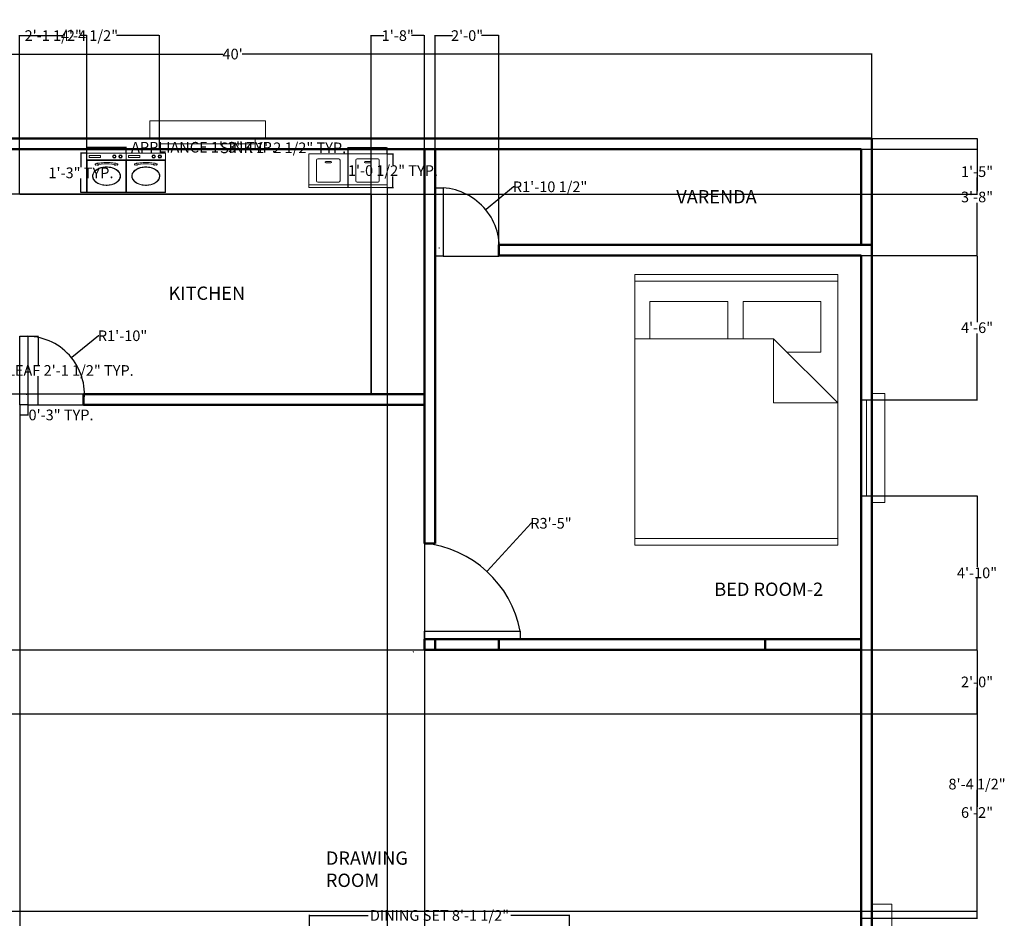
# Model space of a CAD drawing. Units: inches. Extents: x 749 to 1356, y 222 to 907.
# Tile 4 of 4: x 981 to 1351, y 570 to 907. Entities that reach past the tile are written whole.
import ezdxf

# ---------------------------------------------------------------- set-up
doc = ezdxf.new("R2010")
doc.units = ezdxf.units.IN
doc.header["$MEASUREMENT"] = 0
for name, color, linetype, lineweight in [('A-ANNO-DIMS', 30, 'Continuous', 18), ('A-AREA-IDEN', 6, 'Continuous', 25), ('A-EQPM', 8, 'Continuous', 18), ('A-FLOR-CASE', 34, 'Continuous', 25), ('A-FLOR-FIXT', 9, 'Continuous', 18), ('A-GLAZ', 4, 'Continuous', 20), ('A-WALL', 7, 'Continuous', 50), ('DOOR', 4, 'Continuous', 25), ('FURNITURE', 32, 'Continuous', 18)]:
    doc.layers.add(name, color=color, linetype=linetype, lineweight=lineweight)
doc.styles.get("Standard").update_dxf_attribs({"font": 'arial.ttf'})
doc.dimstyles.get("Standard").update_dxf_attribs({"dimtxt": 4, "dimasz": 0.18, "dimexe": 0.18, "dimexo": 0.0625, "dimgap": 0.09, "dimtad": 0, "dimtih": 1, "dimtoh": 1, "dimdec": 0, "dimrnd": 6, "dimzin": 0, "dimdsep": 46, "dimlunit": 3, "dimtxsty": 'Standard', "dimcen": 0.09, "dimadec": 0, "dimazin": 0, "dimtfac": 1, "dimtdec": 0, "dimtofl": 0, "dimtmove": 0, "dimatfit": 3, "dimfxl": 1, "dimtolj": 1, "dimtzin": 0, "dimarcsym": 0})

# ---------------------------------------------------------------- blocks, each defined once
blk = doc.blocks.new('QUEEN-00')
for p, q in [((-0.8475, -0.7751), (-0.8475, 0.7489)), ((0.6511, 0.7489), (0.6511, -0.2925)), ((1.0829, 0.7489), (1.0829, -0.7751)), ((0.9305, 0.6346), (0.6511, 0.6346)), ((0.9305, 0.0504), (0.9305, 0.6346)), ((0.6511, 0.0504), (0.9305, 0.0504)), ((0.9305, -0.0639), (0.6511, -0.0639)), ((0.9305, -0.6481), (0.9305, -0.0639)), ((0.1685, -0.7751), (0.6511, -0.2925)), ((0.1685, -0.2925), (0.1685, -0.7751)), ((0.6511, -0.2925), (0.1685, -0.2925)), ((0.5495, -0.3941), (0.5495, -0.6481)), ((0.5495, -0.6481), (0.9305, -0.6481))]:
    blk.add_line(p, q)
blk.add_lwpolyline([(-0.8983, -0.7751), (-0.8983, 0.7489), (1.1337, 0.7489), (1.1337, -0.7751)], close=True)
blk = doc.blocks.new('A$C7E884C79')
for p, q in [((0, 0), (0, 600)), ((0, 600), (0, 0)), ((0, 600), (600, 600)), ((600, 500), (0, 500)), ((600, 495), (0, 495)), ((600, 600), (600, 0)), ((600, 0), (600, 600)), ((600, 600), (600, 450)), ((600, 600), (600, 500)), ((600, 500), (600, 0)), ((0, 0), (600, 0))]:
    blk.add_line(p, q)
for points in [[(5, 490), (595, 490), (595, 5), (5, 5)], [(36, 565), (209, 565), (209, 535), (36, 535)]]:
    blk.add_lwpolyline(points, close=True)
for centre, radius in [((419, 550), 27), ((419, 550), 17), ((514, 550), 27), ((514, 550), 17)]:
    blk.add_circle(centre, radius)
for centre, radius, start, end in [((137, 428), 10, 107.9829, 276.9581), ((168, 434), 15, 50.7888, 150.367), ((168, 434), 15, 234.0165, 327.1412), ((432, 434), 15, 212.8588, 305.9835), ((432, 434), 15, 29.633, 129.2112), ((463, 428), 10, 263.0419, 72.0171)]:
    blk.add_arc(centre, radius, start, end)
blk.add_ellipse((300, 250), major_axis=(-210, 0), ratio=0.648352)
for points, knots in [([(134, 437), (145, 440), (155, 442), (186, 447), (206, 451), (248, 456), (269, 458), (294, 459), (297, 459), (305, 459), (308, 459), (320, 459), (327, 458), (349, 457), (364, 455), (400, 450), (421, 446), (450, 441), (458, 439), (466, 437)], [0, 0, 0, 0, 31.638865, 31.638865, 92.600143, 92.600143, 153.561421, 153.561421, 164.367647, 164.367647, 175.173874, 175.173874, 196.786327, 196.786327, 240.011233, 240.011233, 302.099201, 302.099201, 326.773065, 326.773065, 326.773065, 326.773065]), ([(85, 250), (85, 245), (86, 240), (88, 227), (90, 219), (96, 205), (100, 198), (110, 184), (116, 177), (128, 165), (135, 159), (151, 148), (159, 143), (177, 134), (187, 130), (206, 123), (217, 120), (238, 115), (249, 113), (271, 110), (282, 109), (305, 109), (316, 109), (339, 111), (350, 113), (372, 117), (382, 120), (403, 126), (412, 130), (431, 138), (440, 143), (456, 153), (464, 159), (478, 170), (484, 177), (495, 190), (499, 197), (507, 211), (510, 219), (513, 234), (514, 241), (515, 256), (514, 264), (510, 279), (508, 287), (500, 301), (496, 308), (486, 321), (480, 328), (466, 340), (459, 345), (442, 356), (434, 361), (415, 369), (405, 373), (385, 380), (375, 382), (353, 387), (342, 388), (320, 390), (308, 391), (286, 391), (275, 390), (252, 388), (241, 386), (220, 381), (209, 378), (189, 371), (180, 367), (162, 358), (153, 353), (138, 342), (130, 337), (117, 324), (112, 318), (102, 304), (98, 297), (91, 283), (89, 275), (86, 262), (85, 256), (85, 250)], [0, 0, 0, 0, 0.108301, 0.108301, 0.267534, 0.267534, 0.426768, 0.426768, 0.586002, 0.586002, 0.745235, 0.745235, 0.904469, 0.904469, 1.063703, 1.063703, 1.222936, 1.222936, 1.38217, 1.38217, 1.541404, 1.541404, 1.700637, 1.700637, 1.859871, 1.859871, 2.019105, 2.019105, 2.178339, 2.178339, 2.337572, 2.337572, 2.496806, 2.496806, 2.65604, 2.65604, 2.815273, 2.815273, 2.974507, 2.974507, 3.133741, 3.133741, 3.292974, 3.292974, 3.452208, 3.452208, 3.611442, 3.611442, 3.770676, 3.770676, 3.929909, 3.929909, 4.089143, 4.089143, 4.248377, 4.248377, 4.40761, 4.40761, 4.566844, 4.566844, 4.726078, 4.726078, 4.885311, 4.885311, 5.044545, 5.044545, 5.203779, 5.203779, 5.363012, 5.363012, 5.522246, 5.522246, 5.68148, 5.68148, 5.840714, 5.840714, 5.999947, 5.999947, 6.159181, 6.159181, 6.283185, 6.283185, 6.283185, 6.283185])]:
    blk.add_open_spline(points, degree=3, knots=knots)
blk.add_open_spline([(138, 418), (192, 428), (300, 449), (408, 428), (462, 418)], degree=3)
blk = doc.blocks.new('LAVAD-01')
for p, q in [((-0.322, 0.358), (-0.322, -0.392)), ((0.328, 0.358), (-0.322, 0.358)), ((-0.272, 0.358), (-0.272, -0.392)), ((0.203, 0.208), (-0.197, 0.208)), ((0.328, -0.392), (0.328, 0.358)), ((-0.222, 0.183), (-0.222, -0.217)), ((0.153, 0.033), (0.153, -0.067)), ((0.165, 0.046), (0.165, 0.046)), ((0.178, -0.067), (0.178, 0.033)), ((0.228, -0.217), (0.228, 0.183)), ((0.165, -0.079), (0.165, -0.079)), ((-0.197, -0.242), (0.203, -0.242)), ((-0.322, -0.392), (0.328, -0.392))]:
    blk.add_line(p, q)
for centre, radius, start, end in [((-0.197, 0.183), 0.025, 90, 180), ((0.203, 0.183), 0.025, 0, 90), ((0.165, 0.033), 0.0125, 90, 180), ((0.165, 0.033), 0.0125, 0, 90), ((0.165, -0.067), 0.0125, 180, 270), ((0.165, -0.067), 0.0125, 270, 360), ((-0.197, -0.217), 0.025, 180, 270), ((0.203, -0.217), 0.025, 270, 360)]:
    blk.add_arc(centre, radius, start, end)
blk = doc.blocks.new('*D129')
at = {"layer": 'A-ANNO-DIMS', "color": 0, "lineweight": -2, "transparency": 16777216}
for p, q in [((820.88, 858.33), (820.88, 894.09)), ((821.06, 893.91), (1057.31, 893.91)), ((1300.7, 893.91), (1064.44, 893.91)), ((1300.88, 862.33), (1300.88, 894.09))]:
    blk.add_line(p, q, dxfattribs=at)
at = {"layer": 'A-ANNO-DIMS', "color": 0, "transparency": 16777216}
for points in [[(821.06, 893.94), (821.06, 893.88), (820.88, 893.91)], [(1300.7, 893.94), (1300.7, 893.88), (1300.88, 893.91)]]:
    blk.add_solid(points, dxfattribs=at)
at = {"layer": 'Defpoints', "color": 0, "transparency": 16777216}
for p in [(1300.88, 893.91), (1300.88, 862.27), (820.88, 858.27)]:
    blk.add_point(p, dxfattribs=at)
at = {"layer": 'A-ANNO-DIMS', "color": 0, "transparency": 16777216, "insert": (1060.88, 893.91), "char_height": 4, "attachment_point": 5}
blk.add_mtext("\\A1;40'", dxfattribs=at)
blk = doc.blocks.new('WIN-36IN')
blk.add_lwpolyline([(0, 0), (0, 36), (4, 36), (4, 0)], close=True)
blk.add_lwpolyline([(4, 0), (2.02, 0), (2.02, 36)])
blk = doc.blocks.new('DOOR-LEAF-36IN')
blk.add_lwpolyline([(0, 3), (36, 3), (36, 0), (0, 0)], close=True)
blk = doc.blocks.new('DOOR-LEAF-NARROW')
blk.add_line((0, 25.67), (3, 25.67))
blk.add_lwpolyline([(3, 25.67), (3, 0), (0, 0), (0, 25.67)])
blk = doc.blocks.new('*D141')
at = {"layer": 'A-ANNO-DIMS', "color": 0, "lineweight": -2, "transparency": 16777216}
for p, q in [((984.05, 787.99), (988.01, 787.99)), ((987.83, 787.81), (987.83, 777.32)), ((987.83, 762.5), (987.83, 773)), ((984.05, 762.32), (988.01, 762.32))]:
    blk.add_line(p, q, dxfattribs=at)
at = {"layer": 'A-ANNO-DIMS', "color": 0, "transparency": 16777216}
for points in [[(987.8, 787.81), (987.86, 787.81), (987.83, 787.99)], [(987.8, 762.5), (987.86, 762.5), (987.83, 762.32)]]:
    blk.add_solid(points, dxfattribs=at)
at = {"layer": 'Defpoints', "color": 0, "transparency": 16777216}
for p in [(983.98, 787.99), (987.83, 787.99), (983.98, 762.32)]:
    blk.add_point(p, dxfattribs=at)
at = {"layer": 'A-ANNO-DIMS', "color": 0, "transparency": 16777216, "insert": (987.83, 775.16), "char_height": 4, "attachment_point": 5}
blk.add_mtext('\\A1;NARROW LEAF 2\'-1 1/2" TYP.', dxfattribs=at)
blk = doc.blocks.new('*D142')
at = {"layer": 'A-ANNO-DIMS', "color": 0, "lineweight": -2, "transparency": 16777216}
for p, q in [((980.98, 762.26), (980.98, 758.29)), ((983.98, 762.26), (983.98, 758.29)), ((981.16, 758.47), (983.8, 758.47)), ((983.98, 758.47), (984.16, 758.47))]:
    blk.add_line(p, q, dxfattribs=at)
at = {"layer": 'A-ANNO-DIMS', "color": 0, "transparency": 16777216}
for points in [[(981.16, 758.5), (981.16, 758.44), (980.98, 758.47)], [(983.8, 758.5), (983.8, 758.44), (983.98, 758.47)]]:
    blk.add_solid(points, dxfattribs=at)
at = {"layer": 'Defpoints', "color": 0, "transparency": 16777216}
for p in [(980.98, 762.32), (983.98, 762.32), (983.98, 758.47)]:
    blk.add_point(p, dxfattribs=at)
at = {"layer": 'A-ANNO-DIMS', "color": 0, "transparency": 16777216, "insert": (996.45, 758.47), "char_height": 4, "attachment_point": 5}
blk.add_mtext('\\A1;0\'-3" TYP.', dxfattribs=at)
blk = doc.blocks.new('*D145')
at = {"layer": 'A-ANNO-DIMS', "color": 0, "lineweight": -2, "transparency": 16777216}
for p, q in [((1104.24, 858.72), (1104.06, 858.72)), ((1104.24, 856.58), (1104.24, 858.9)), ((1118.7, 858.72), (1104.42, 858.72)), ((1118.88, 856.58), (1118.88, 858.9))]:
    blk.add_line(p, q, dxfattribs=at)
at = {"layer": 'A-ANNO-DIMS', "color": 0, "transparency": 16777216}
for points in [[(1104.42, 858.75), (1104.42, 858.69), (1104.24, 858.72)], [(1118.7, 858.75), (1118.7, 858.69), (1118.88, 858.72)]]:
    blk.add_solid(points, dxfattribs=at)
at = {"layer": 'Defpoints', "color": 0, "transparency": 16777216}
for p in [(1104.24, 858.72), (1104.24, 856.52), (1118.88, 856.52)]:
    blk.add_point(p, dxfattribs=at)
at = {"layer": 'A-ANNO-DIMS', "color": 0, "transparency": 16777216, "insert": (1079.83, 858.72), "char_height": 4, "attachment_point": 5}
blk.add_mtext('\\A1;SINK 1\'-2 1/2" TYP.', dxfattribs=at)
blk = doc.blocks.new('*D146')
at = {"layer": 'A-ANNO-DIMS', "color": 0, "lineweight": -2, "transparency": 16777216}
for p, q in [((1118.95, 856.52), (1121.26, 856.52)), ((1121.08, 856.34), (1121.08, 852.34)), ((1121.08, 844.01), (1121.08, 848.02)), ((1118.95, 843.83), (1121.26, 843.83))]:
    blk.add_line(p, q, dxfattribs=at)
at = {"layer": 'A-ANNO-DIMS', "color": 0, "transparency": 16777216}
for points in [[(1121.05, 856.34), (1121.11, 856.34), (1121.08, 856.52)], [(1121.05, 844.01), (1121.11, 844.01), (1121.08, 843.83)]]:
    blk.add_solid(points, dxfattribs=at)
at = {"layer": 'Defpoints', "color": 0, "transparency": 16777216}
for p in [(1118.88, 856.52), (1121.08, 856.52), (1118.88, 843.83)]:
    blk.add_point(p, dxfattribs=at)
at = {"layer": 'A-ANNO-DIMS', "color": 0, "transparency": 16777216, "insert": (1121.08, 850.18), "char_height": 4, "attachment_point": 5}
blk.add_mtext('\\A1;1\'-0 1/2" TYP.', dxfattribs=at)
blk = doc.blocks.new('*D149')
at = {"layer": 'A-ANNO-DIMS', "color": 0, "lineweight": -2, "transparency": 16777216}
for p, q in [((1006.14, 856.78), (1006.14, 859.11)), ((1006.32, 858.93), (1020.72, 858.93)), ((1020.9, 856.78), (1020.9, 859.11)), ((1020.9, 858.93), (1021.08, 858.93))]:
    blk.add_line(p, q, dxfattribs=at)
at = {"layer": 'A-ANNO-DIMS', "color": 0, "transparency": 16777216}
for points in [[(1006.32, 858.96), (1006.32, 858.9), (1006.14, 858.93)], [(1020.72, 858.96), (1020.72, 858.9), (1020.9, 858.93)]]:
    blk.add_solid(points, dxfattribs=at)
at = {"layer": 'Defpoints', "color": 0, "transparency": 16777216}
for p in [(1020.9, 858.93), (1006.14, 856.71), (1020.9, 856.71)]:
    blk.add_point(p, dxfattribs=at)
at = {"layer": 'A-ANNO-DIMS', "color": 0, "transparency": 16777216, "insert": (1049.94, 858.93), "char_height": 4, "attachment_point": 5}
blk.add_mtext('\\A1;APPLIANCE 1\'-3" TYP.', dxfattribs=at)
blk = doc.blocks.new('*D150')
at = {"layer": 'A-ANNO-DIMS', "color": 0, "lineweight": -2, "transparency": 16777216}
for p, q in [((1006.08, 856.71), (1003.75, 856.71)), ((1003.93, 856.53), (1003.93, 851.47)), ((1003.93, 842.13), (1003.93, 847.2)), ((1006.08, 841.95), (1003.75, 841.95))]:
    blk.add_line(p, q, dxfattribs=at)
at = {"layer": 'A-ANNO-DIMS', "color": 0, "transparency": 16777216}
for points in [[(1003.9, 856.53), (1003.96, 856.53), (1003.93, 856.71)], [(1003.9, 842.13), (1003.96, 842.13), (1003.93, 841.95)]]:
    blk.add_solid(points, dxfattribs=at)
at = {"layer": 'Defpoints', "color": 0, "transparency": 16777216}
for p in [(1003.93, 856.71), (1006.14, 856.71), (1006.14, 841.95)]:
    blk.add_point(p, dxfattribs=at)
at = {"layer": 'A-ANNO-DIMS', "color": 0, "transparency": 16777216, "insert": (1003.93, 849.33), "char_height": 4, "attachment_point": 5}
blk.add_mtext('\\A1;1\'-3" TYP.', dxfattribs=at)
blk = doc.blocks.new('*D151')
at = {"layer": 'A-ANNO-DIMS', "color": 0, "lineweight": -2, "transparency": 16777216}
for p, q in [((1089.75, 556.06), (1089.75, 570.82)), ((1089.93, 570.64), (1111.83, 570.64)), ((1187.2, 570.64), (1165.29, 570.64)), ((1187.38, 556.06), (1187.38, 570.82))]:
    blk.add_line(p, q, dxfattribs=at)
at = {"layer": 'A-ANNO-DIMS', "color": 0, "transparency": 16777216}
for points in [[(1089.93, 570.67), (1089.93, 570.61), (1089.75, 570.64)], [(1187.2, 570.67), (1187.2, 570.61), (1187.38, 570.64)]]:
    blk.add_solid(points, dxfattribs=at)
at = {"layer": 'Defpoints', "color": 0, "transparency": 16777216}
for p in [(1187.38, 570.64), (1089.75, 556), (1187.38, 556)]:
    blk.add_point(p, dxfattribs=at)
at = {"layer": 'A-ANNO-DIMS', "color": 0, "transparency": 16777216, "insert": (1138.56, 570.64), "char_height": 4, "attachment_point": 5}
blk.add_mtext('\\A1;DINING SET 8\'-1 1/2"', dxfattribs=at)
blk = doc.blocks.new('*D163')
at = {"layer": 'A-ANNO-DIMS', "color": 0, "lineweight": -2, "transparency": 16777216}
for p, q in [((1296.94, 670.27), (1340.58, 670.27)), ((1340.4, 670.09), (1340.4, 622.07)), ((1340.4, 569.75), (1340.4, 617.76)), ((1296.93, 569.57), (1340.58, 569.57))]:
    blk.add_line(p, q, dxfattribs=at)
at = {"layer": 'A-ANNO-DIMS', "color": 0, "transparency": 16777216}
for points in [[(1340.37, 670.09), (1340.43, 670.09), (1340.4, 670.27)], [(1340.37, 569.75), (1340.43, 569.75), (1340.4, 569.57)]]:
    blk.add_solid(points, dxfattribs=at)
at = {"layer": 'Defpoints', "color": 0, "transparency": 16777216}
for p in [(1296.88, 670.27), (1340.4, 670.27), (1296.87, 569.57)]:
    blk.add_point(p, dxfattribs=at)
at = {"layer": 'A-ANNO-DIMS', "color": 0, "transparency": 16777216, "insert": (1340.4, 619.92), "char_height": 4, "attachment_point": 5}
blk.add_mtext('\\A1;8\'-4 1/2"', dxfattribs=at)
blk = doc.blocks.new('*D164')
at = {"layer": 'A-ANNO-DIMS', "color": 0, "lineweight": -2, "transparency": 16777216}
for p, q in [((1296.96, 728.15), (1340.58, 728.15)), ((1340.4, 727.97), (1340.4, 701.34)), ((1340.4, 670.45), (1340.4, 697.07)), ((1296.94, 670.27), (1340.58, 670.27))]:
    blk.add_line(p, q, dxfattribs=at)
at = {"layer": 'A-ANNO-DIMS', "color": 0, "transparency": 16777216}
for points in [[(1340.37, 727.97), (1340.43, 727.97), (1340.4, 728.15)], [(1340.37, 670.45), (1340.43, 670.45), (1340.4, 670.27)]]:
    blk.add_solid(points, dxfattribs=at)
at = {"layer": 'Defpoints', "color": 0, "transparency": 16777216}
for p in [(1296.9, 728.15), (1340.4, 728.15), (1296.88, 670.27)]:
    blk.add_point(p, dxfattribs=at)
at = {"layer": 'A-ANNO-DIMS', "color": 0, "transparency": 16777216, "insert": (1340.4, 699.21), "char_height": 4, "attachment_point": 5}
blk.add_mtext('\\A1;4\'-10"', dxfattribs=at)
blk = doc.blocks.new('*D165')
at = {"layer": 'A-ANNO-DIMS', "color": 0, "lineweight": -2, "transparency": 16777216}
for p, q in [((1296.94, 818.27), (1340.58, 818.27)), ((1340.4, 818.09), (1340.4, 793.34)), ((1340.4, 764.33), (1340.4, 789.07)), ((1296.96, 764.15), (1340.58, 764.15))]:
    blk.add_line(p, q, dxfattribs=at)
at = {"layer": 'A-ANNO-DIMS', "color": 0, "transparency": 16777216}
for points in [[(1340.37, 818.09), (1340.43, 818.09), (1340.4, 818.27)], [(1340.37, 764.33), (1340.43, 764.33), (1340.4, 764.15)]]:
    blk.add_solid(points, dxfattribs=at)
at = {"layer": 'Defpoints', "color": 0, "transparency": 16777216}
for p in [(1296.88, 818.27), (1340.4, 818.27), (1296.9, 764.15)]:
    blk.add_point(p, dxfattribs=at)
at = {"layer": 'A-ANNO-DIMS', "color": 0, "transparency": 16777216, "insert": (1340.4, 791.21), "char_height": 4, "attachment_point": 5}
blk.add_mtext('\\A1;4\'-6"', dxfattribs=at)
blk = doc.blocks.new('*D166')
at = {"layer": 'A-ANNO-DIMS', "color": 0, "lineweight": -2, "transparency": 16777216}
for p, q in [((1300.94, 862.27), (1340.58, 862.27)), ((1340.4, 862.09), (1340.4, 842.4)), ((1340.4, 818.45), (1340.4, 838.13)), ((1296.94, 818.27), (1340.58, 818.27))]:
    blk.add_line(p, q, dxfattribs=at)
at = {"layer": 'A-ANNO-DIMS', "color": 0, "transparency": 16777216}
for points in [[(1340.37, 862.09), (1340.43, 862.09), (1340.4, 862.27)], [(1340.37, 818.45), (1340.43, 818.45), (1340.4, 818.27)]]:
    blk.add_solid(points, dxfattribs=at)
at = {"layer": 'Defpoints', "color": 0, "transparency": 16777216}
for p in [(1300.88, 862.27), (1340.4, 862.27), (1296.88, 818.27)]:
    blk.add_point(p, dxfattribs=at)
at = {"layer": 'A-ANNO-DIMS', "color": 0, "transparency": 16777216, "insert": (1340.4, 840.27), "char_height": 4, "attachment_point": 5}
blk.add_mtext('\\A1;3\'-8"', dxfattribs=at)
blk = doc.blocks.new('*D169')
at = {"layer": 'A-ANNO-DIMS', "color": 0, "lineweight": -2, "transparency": 16777216}
for p, q in [((980.88, 858.33), (980.88, 901.02)), ((981.06, 900.84), (997, 900.84)), ((1033.23, 900.84), (1017.29, 900.84)), ((1033.41, 858.31), (1033.41, 901.02))]:
    blk.add_line(p, q, dxfattribs=at)
at = {"layer": 'A-ANNO-DIMS', "color": 0, "transparency": 16777216}
for points in [[(981.06, 900.87), (981.06, 900.81), (980.88, 900.84)], [(1033.23, 900.87), (1033.23, 900.81), (1033.41, 900.84)]]:
    blk.add_solid(points, dxfattribs=at)
at = {"layer": 'Defpoints', "color": 0, "transparency": 16777216}
for p in [(1033.41, 900.84), (980.88, 858.27), (1033.41, 858.25)]:
    blk.add_point(p, dxfattribs=at)
at = {"layer": 'A-ANNO-DIMS', "color": 0, "transparency": 16777216, "insert": (1007.14, 900.84), "char_height": 4, "attachment_point": 5}
blk.add_mtext('\\A1;4\'-4 1/2"', dxfattribs=at)
blk = doc.blocks.new('*D174')
at = {"layer": 'A-ANNO-DIMS', "color": 0, "lineweight": -2, "transparency": 16777216}
for p, q in [((900.94, 646.27), (1340.58, 646.27)), ((1340.4, 646.09), (1340.4, 611.4)), ((1340.4, 572.45), (1340.4, 607.13)), ((896.94, 572.27), (1340.58, 572.27))]:
    blk.add_line(p, q, dxfattribs=at)
at = {"layer": 'A-ANNO-DIMS', "color": 0, "transparency": 16777216}
for points in [[(1340.37, 646.09), (1340.43, 646.09), (1340.4, 646.27)], [(1340.37, 572.45), (1340.43, 572.45), (1340.4, 572.27)]]:
    blk.add_solid(points, dxfattribs=at)
at = {"layer": 'Defpoints', "color": 0, "transparency": 16777216}
for p in [(900.88, 646.27), (1340.4, 646.27), (896.88, 572.27)]:
    blk.add_point(p, dxfattribs=at)
at = {"layer": 'A-ANNO-DIMS', "color": 0, "transparency": 16777216, "insert": (1340.4, 609.27), "char_height": 4, "attachment_point": 5}
blk.add_mtext('\\A1;6\'-2"', dxfattribs=at)
blk = doc.blocks.new('*D175')
at = {"layer": 'A-ANNO-DIMS', "color": 0, "lineweight": -2, "transparency": 16777216}
for p, q in [((900.94, 670.27), (1340.58, 670.27)), ((1340.4, 670.09), (1340.4, 660.4)), ((1340.4, 646.45), (1340.4, 656.13)), ((900.94, 646.27), (1340.58, 646.27))]:
    blk.add_line(p, q, dxfattribs=at)
at = {"layer": 'A-ANNO-DIMS', "color": 0, "transparency": 16777216}
for points in [[(1340.37, 670.09), (1340.43, 670.09), (1340.4, 670.27)], [(1340.37, 646.45), (1340.43, 646.45), (1340.4, 646.27)]]:
    blk.add_solid(points, dxfattribs=at)
at = {"layer": 'Defpoints', "color": 0, "transparency": 16777216}
for p in [(900.88, 670.27), (1340.4, 670.27), (900.88, 646.27)]:
    blk.add_point(p, dxfattribs=at)
at = {"layer": 'A-ANNO-DIMS', "color": 0, "transparency": 16777216, "insert": (1340.4, 658.27), "char_height": 4, "attachment_point": 5}
blk.add_mtext('\\A1;2\'-0"', dxfattribs=at)
blk = doc.blocks.new('*D179')
at = {"layer": 'A-ANNO-DIMS', "color": 0, "lineweight": -2, "transparency": 16777216}
for p, q in [((1112.81, 841.27), (760.48, 841.27)), ((760.66, 841.09), (760.66, 805.9)), ((760.66, 766.45), (760.66, 801.63)), ((1112.81, 766.27), (760.48, 766.27))]:
    blk.add_line(p, q, dxfattribs=at)
at = {"layer": 'A-ANNO-DIMS', "color": 0, "transparency": 16777216}
for points in [[(760.63, 841.09), (760.69, 841.09), (760.66, 841.27)], [(760.63, 766.45), (760.69, 766.45), (760.66, 766.27)]]:
    blk.add_solid(points, dxfattribs=at)
at = {"layer": 'Defpoints', "color": 0, "transparency": 16777216}
for p in [(760.66, 841.27), (1112.88, 841.27), (1112.88, 766.27)]:
    blk.add_point(p, dxfattribs=at)
at = {"layer": 'A-ANNO-DIMS', "color": 0, "transparency": 16777216, "insert": (760.66, 803.77), "char_height": 4, "attachment_point": 5}
blk.add_mtext('\\A1;6\'-3"', dxfattribs=at)
blk = doc.blocks.new('*D180')
at = {"layer": 'A-ANNO-DIMS', "color": 0, "lineweight": -2, "transparency": 16777216}
for p, q in [((980.98, 762.26), (980.98, 224.8)), ((1132.88, 762.2), (1132.88, 224.8)), ((981.16, 224.98), (1050.16, 224.98)), ((1132.7, 224.98), (1063.7, 224.98))]:
    blk.add_line(p, q, dxfattribs=at)
at = {"layer": 'A-ANNO-DIMS', "color": 0, "transparency": 16777216}
for points in [[(981.16, 225.01), (981.16, 224.95), (980.98, 224.98)], [(1132.7, 225.01), (1132.7, 224.95), (1132.88, 224.98)]]:
    blk.add_solid(points, dxfattribs=at)
at = {"layer": 'Defpoints', "color": 0, "transparency": 16777216}
for p in [(980.98, 762.32), (1132.88, 762.27), (1132.88, 224.98)]:
    blk.add_point(p, dxfattribs=at)
at = {"layer": 'A-ANNO-DIMS', "color": 0, "transparency": 16777216, "insert": (1056.93, 224.98), "char_height": 4, "attachment_point": 5}
blk.add_mtext('\\A1;12\'-8"', dxfattribs=at)
blk = doc.blocks.new('*D181')
at = {"layer": 'A-ANNO-DIMS', "color": 0, "lineweight": -2, "transparency": 16777216}
for p, q in [((1112.88, 766.33), (1112.88, 901.02)), ((1113.06, 900.84), (1117.66, 900.84)), ((1132.7, 900.84), (1128.1, 900.84)), ((1132.88, 766.33), (1132.88, 901.02))]:
    blk.add_line(p, q, dxfattribs=at)
at = {"layer": 'A-ANNO-DIMS', "color": 0, "transparency": 16777216}
for points in [[(1113.06, 900.87), (1113.06, 900.81), (1112.88, 900.84)], [(1132.7, 900.87), (1132.7, 900.81), (1132.88, 900.84)]]:
    blk.add_solid(points, dxfattribs=at)
at = {"layer": 'Defpoints', "color": 0, "transparency": 16777216}
for p in [(1132.88, 900.84), (1112.88, 766.27), (1132.88, 766.27)]:
    blk.add_point(p, dxfattribs=at)
at = {"layer": 'A-ANNO-DIMS', "color": 0, "transparency": 16777216, "insert": (1122.88, 900.84), "char_height": 4, "attachment_point": 5}
blk.add_mtext('\\A1;1\'-8"', dxfattribs=at)
blk = doc.blocks.new('*D182')
at = {"layer": 'A-ANNO-DIMS', "color": 0, "lineweight": -2, "transparency": 16777216}
for p, q in [((980.94, 858.27), (1340.58, 858.27)), ((1340.4, 858.09), (1340.4, 851.9)), ((1340.4, 841.45), (1340.4, 847.63)), ((980.94, 841.27), (1340.58, 841.27))]:
    blk.add_line(p, q, dxfattribs=at)
at = {"layer": 'A-ANNO-DIMS', "color": 0, "transparency": 16777216}
for points in [[(1340.37, 858.09), (1340.43, 858.09), (1340.4, 858.27)], [(1340.37, 841.45), (1340.43, 841.45), (1340.4, 841.27)]]:
    blk.add_solid(points, dxfattribs=at)
at = {"layer": 'Defpoints', "color": 0, "transparency": 16777216}
for p in [(980.88, 858.27), (1340.4, 858.27), (980.88, 841.27)]:
    blk.add_point(p, dxfattribs=at)
at = {"layer": 'A-ANNO-DIMS', "color": 0, "transparency": 16777216, "insert": (1340.4, 849.77), "char_height": 4, "attachment_point": 5}
blk.add_mtext('\\A1;1\'-5"', dxfattribs=at)
blk = doc.blocks.new('*D184')
at = {"layer": 'A-ANNO-DIMS', "color": 0, "lineweight": -2, "transparency": 16777216}
for p, q in [((980.88, 841.33), (980.88, 901.02)), ((981.06, 900.84), (983.41, 900.84)), ((1005.96, 900.84), (1003.61, 900.84)), ((1006.14, 842.02), (1006.14, 901.02))]:
    blk.add_line(p, q, dxfattribs=at)
at = {"layer": 'A-ANNO-DIMS', "color": 0, "transparency": 16777216}
for points in [[(981.06, 900.87), (981.06, 900.81), (980.88, 900.84)], [(1005.96, 900.87), (1005.96, 900.81), (1006.14, 900.84)]]:
    blk.add_solid(points, dxfattribs=at)
at = {"layer": 'Defpoints', "color": 0, "transparency": 16777216}
for p in [(1006.14, 900.84), (980.88, 841.27), (1006.14, 841.95)]:
    blk.add_point(p, dxfattribs=at)
at = {"layer": 'A-ANNO-DIMS', "color": 0, "transparency": 16777216, "insert": (993.51, 900.84), "char_height": 4, "attachment_point": 5}
blk.add_mtext('\\A1;2\'-1 1/2"', dxfattribs=at)
blk = doc.blocks.new('*D185')
at = {"layer": 'A-ANNO-DIMS', "color": 0, "lineweight": -2, "transparency": 16777216}
for p, q in [((1132.88, 858.2), (1132.88, 224.8)), ((1118.88, 843.77), (1118.88, 224.8)), ((1119.06, 224.98), (1120.66, 224.98)), ((1132.7, 224.98), (1131.1, 224.98))]:
    blk.add_line(p, q, dxfattribs=at)
at = {"layer": 'A-ANNO-DIMS', "color": 0, "transparency": 16777216}
for points in [[(1119.06, 225.01), (1119.06, 224.95), (1118.88, 224.98)], [(1132.7, 225.01), (1132.7, 224.95), (1132.88, 224.98)]]:
    blk.add_solid(points, dxfattribs=at)
at = {"layer": 'Defpoints', "color": 0, "transparency": 16777216}
for p in [(1132.88, 858.27), (1118.88, 843.83), (1132.88, 224.98)]:
    blk.add_point(p, dxfattribs=at)
at = {"layer": 'A-ANNO-DIMS', "color": 0, "transparency": 16777216, "insert": (1125.88, 224.98), "char_height": 4, "attachment_point": 5}
blk.add_mtext('\\A1;1\'-2"', dxfattribs=at)
blk = doc.blocks.new('*D187')
at = {"layer": 'A-ANNO-DIMS', "color": 0, "lineweight": -2, "transparency": 16777216}
for p, q in [((1136.96, 818.07), (1136.96, 901.02)), ((1137.14, 900.84), (1143.48, 900.84)), ((1160.7, 900.84), (1154.36, 900.84)), ((1160.88, 822.33), (1160.88, 901.02))]:
    blk.add_line(p, q, dxfattribs=at)
at = {"layer": 'A-ANNO-DIMS', "color": 0, "transparency": 16777216}
for points in [[(1137.14, 900.87), (1137.14, 900.81), (1136.96, 900.84)], [(1160.7, 900.87), (1160.7, 900.81), (1160.88, 900.84)]]:
    blk.add_solid(points, dxfattribs=at)
at = {"layer": 'Defpoints', "color": 0, "transparency": 16777216}
for p in [(1160.88, 900.84), (1160.88, 822.27), (1136.96, 818)]:
    blk.add_point(p, dxfattribs=at)
at = {"layer": 'A-ANNO-DIMS', "color": 0, "transparency": 16777216, "insert": (1148.92, 900.84), "char_height": 4, "attachment_point": 5}
blk.add_mtext('\\A1;2\'-0"', dxfattribs=at)
blk = doc.blocks.new('*D192')
at = {"layer": 'A-ANNO-DIMS', "color": 0, "lineweight": -2, "transparency": 16777216}
for p, q in [((1172.92, 717.81), (1156.47, 699.87)), ((1173.1, 717.81), (1172.92, 717.81)), ((1128.65, 669.61), (1128.83, 669.61)), ((1128.74, 669.52), (1128.74, 669.7))]:
    blk.add_line(p, q, dxfattribs=at)
at = {"layer": 'A-ANNO-DIMS', "color": 0, "transparency": 16777216}
blk.add_solid([(1156.45, 699.89), (1156.49, 699.85), (1156.35, 699.74)], dxfattribs=at)
at = {"layer": 'Defpoints', "color": 0, "transparency": 16777216}
for p in [(1156.35, 699.74), (1128.74, 669.61)]:
    blk.add_point(p, dxfattribs=at)
at = {"layer": 'A-ANNO-DIMS', "color": 0, "transparency": 16777216, "insert": (1180.42, 717.81), "char_height": 4, "attachment_point": 5}
blk.add_mtext('\\A1;R3\'-5"', dxfattribs=at)
blk = doc.blocks.new('*D201')
at = {"layer": 'A-ANNO-DIMS', "color": 0, "lineweight": -2, "transparency": 16777216}
for p, q in [((1166.37, 844.1), (1156.05, 835.61)), ((1166.55, 844.1), (1166.37, 844.1)), ((1138.39, 821.14), (1138.57, 821.14)), ((1138.48, 821.05), (1138.48, 821.23))]:
    blk.add_line(p, q, dxfattribs=at)
at = {"layer": 'A-ANNO-DIMS', "color": 0, "transparency": 16777216}
blk.add_solid([(1156.03, 835.63), (1156.07, 835.58), (1155.91, 835.49)], dxfattribs=at)
at = {"layer": 'Defpoints', "color": 0, "transparency": 16777216}
for p in [(1155.91, 835.49), (1138.48, 821.14)]:
    blk.add_point(p, dxfattribs=at)
at = {"layer": 'A-ANNO-DIMS', "color": 0, "transparency": 16777216, "insert": (1180.09, 844.1), "char_height": 4, "attachment_point": 5}
blk.add_mtext('\\A1;R1\'-10 1/2"', dxfattribs=at)
blk = doc.blocks.new('*D202')
at = {"layer": 'A-ANNO-DIMS', "color": 0, "lineweight": -2, "transparency": 16777216}
for p, q in [((1010.51, 788.19), (1000.51, 780.07)), ((1010.69, 788.19), (1010.51, 788.19)), ((983.39, 766.23), (983.57, 766.23)), ((983.48, 766.14), (983.48, 766.32))]:
    blk.add_line(p, q, dxfattribs=at)
at = {"layer": 'A-ANNO-DIMS', "color": 0, "transparency": 16777216}
blk.add_solid([(1000.49, 780.09), (1000.53, 780.04), (1000.37, 779.95)], dxfattribs=at)
at = {"layer": 'Defpoints', "color": 0, "transparency": 16777216}
for p in [(1000.37, 779.95), (983.48, 766.23)]:
    blk.add_point(p, dxfattribs=at)
at = {"layer": 'A-ANNO-DIMS', "color": 0, "transparency": 16777216, "insert": (1019.56, 788.19), "char_height": 4, "attachment_point": 5}
blk.add_mtext('\\A1;R1\'-10"', dxfattribs=at)

msp = doc.modelspace()

# ---------------------------------------------------------------- linework, layer by layer
at = {"layer": 'A-FLOR-CASE'}
for q in [(980.88, 841.27), (1112.88, 766.27)]:
    msp.add_line((1112.88, 841.27), q, dxfattribs=at)
at = {"layer": 'A-GLAZ'}
for p, q in [((1029.83, 868.79), (1073.28, 868.79)), ((1029.83, 862.27), (1029.83, 868.79)), ((1073.28, 868.79), (1073.28, 862.27)), ((1300.88, 766.48), (1305.77, 766.48)), ((1305.77, 766.48), (1305.77, 725.58)), ((1305.77, 725.58), (1300.88, 725.58)), ((1300.88, 574.82), (1308.35, 574.82)), ((1308.35, 574.82), (1308.35, 529.73))]:
    msp.add_line(p, q, dxfattribs=at)
at = {"layer": 'A-WALL'}
for p, q in [((1300.88, 862.27), (820.88, 862.27)), ((1300.88, 466.27), (1300.88, 862.27)), ((1296.88, 858.27), (824.88, 858.27)), ((1132.88, 858.27), (1132.88, 710.27)), ((1136.88, 858.27), (1136.88, 710.27)), ((1296.88, 822.27), (1296.88, 858.27)), ((1300.88, 822.27), (1160.88, 822.27)), ((1160.88, 822.27), (1160.88, 818.27)), ((1296.88, 818.27), (1160.88, 818.27)), ((1296.88, 466.27), (1296.88, 818.27)), ((1132.88, 766.27), (1004.88, 766.27)), ((1004.88, 766.27), (1004.88, 762.27)), ((1132.88, 762.27), (1004.88, 762.27)), ((1136.88, 710.27), (1132.88, 710.27)), ((1296.88, 674.27), (1132.88, 674.27)), ((1132.88, 674.27), (1132.88, 670.27)), ((1136.88, 674.27), (1136.88, 670.27)), ((1160.88, 674.27), (1160.88, 670.27)), ((1260.88, 670.27), (1260.88, 674.27)), ((1296.88, 670.27), (1132.88, 670.27))]:
    msp.add_line(p, q, dxfattribs=at)
at = {"layer": 'DOOR'}
for p, q in [((1139.96, 818), (1160.84, 818)), ((983.98, 762.32), (1004.88, 762.27)), ((1132.88, 710.27), (1132.88, 677.27))]:
    msp.add_line(p, q, dxfattribs=at)
for centre, radius, start, end in [((1138.48, 821.14), 22.58, 352.6839, 86.2478), ((983.48, 766.23), 21.77, 349.5084, 88.659), ((1128.74, 669.61), 40.87, 10.7963, 84.1828)]:
    msp.add_arc(centre, radius, start, end, dxfattribs=at)

# ---------------------------------------------------------------- block references
at = {"layer": 'A-EQPM', "xscale": 0.0245997790988797, "yscale": 0.0245997790988797, "zscale": 0.0245997790988797}
for p in [(1006.14, 841.95), (1020.9, 841.95)]:
    msp.add_blockref('A$C7E884C79', p, dxfattribs=at)
at = {"layer": 'A-FLOR-FIXT', "xscale": 19.52304203340109, "yscale": 19.52304203340109, "zscale": 19.52304203340109, "rotation": 90}
for p in [(1096.48, 850.12), (1111.24, 850.12)]:
    msp.add_blockref('LAVAD-01', p, dxfattribs=at)
at = {"layer": 'A-GLAZ', "rotation": 269.9999999999997}
msp.add_blockref('WIN-36IN', (1033.41, 862.24), dxfattribs=at)
at = {"layer": 'A-GLAZ'}
msp.add_blockref('WIN-36IN', (1296.9, 728.15), dxfattribs=at)
at = {"layer": 'DOOR'}
for p in [(1136.96, 818), (980.98, 762.32)]:
    msp.add_blockref('DOOR-LEAF-NARROW', p, dxfattribs=at)
at = {"layer": 'DOOR', "rotation": 180}
msp.add_blockref('DOOR-LEAF-36IN', (1168.88, 677.27), dxfattribs=at)
at = {"layer": 'FURNITURE', "xscale": 49.9999999999977, "yscale": 49.9999999999977, "zscale": 49.9999999999977, "rotation": 90}
msp.add_blockref('QUEEN-00', (1249.33, 754.53), dxfattribs=at)

# ---------------------------------------------------------------- texts
at = {"layer": 'A-AREA-IDEN', "char_height": 5, "attachment_point": 1}
for s, insert in [('VARENDA', (1227.47, 842.86)), ('KITCHEN', (1036.83, 806.66)), ('BED ROOM-2', (1241.74, 695.55)), ('DRAWING ROOM', (1095.9, 594.66))]:
    msp.add_mtext_dynamic_manual_height_columns(s, width=49.3334, gutter_width=1, heights=[0], dxfattribs=dict(at, insert=insert))

# ---------------------------------------------------------------- dimensions: what is measured, and where the dimension line sits
at = {"layer": 'A-ANNO-DIMS'}
for base, p1, p2, override, picture, middle in [((1033.41, 900.84), (980.88, 858.27), (1033.41, 858.25), {"dimdec": 1, "dimlfac": 1, "dimrnd": 0, "dimzin": 1, "dimdsep": 46, "dimlunit": 4, "dimfrac": 2}, '*D169', (1007.14, 900.84)), ((1006.14, 900.84), (980.88, 841.27), (1006.14, 841.95), {"dimdec": 1, "dimlfac": 1, "dimrnd": 0, "dimzin": 1, "dimdsep": 46, "dimlunit": 4, "dimfrac": 2}, '*D184', (993.51, 900.84)), ((1132.88, 900.84), (1112.88, 766.27), (1132.88, 766.27), {"dimdec": 1, "dimlfac": 1, "dimrnd": 0, "dimzin": 1, "dimdsep": 46, "dimlunit": 4, "dimfrac": 2}, '*D181', (1122.88, 900.84)), ((1160.88, 900.84), (1136.96, 818), (1160.88, 822.27), {"dimdec": 1, "dimlfac": 1, "dimrnd": 0, "dimzin": 1, "dimdsep": 46, "dimlunit": 4, "dimfrac": 2}, '*D187', (1148.92, 900.84)), ((1300.88, 893.91), (820.88, 858.27), (1300.88, 862.27), {"dimclrd": 0, "dimclre": 0, "dimclrt": 0}, '*D129', (1060.88, 893.91)), ((1132.88, 224.98), (1118.88, 843.83), (1132.88, 858.27), {"dimdec": 1, "dimlfac": 1, "dimrnd": 0, "dimzin": 1, "dimdsep": 46, "dimlunit": 4, "dimfrac": 2}, '*D185', (1125.88, 224.98)), ((1132.88, 224.98), (980.98, 762.32), (1132.88, 762.27), {"dimdec": 1, "dimlfac": 1, "dimrnd": 0, "dimzin": 1, "dimdsep": 46, "dimlunit": 4, "dimfrac": 2}, '*D180', (1056.93, 224.98))]:
    dim = msp.add_linear_dim(base=base, p1=p1, p2=p2, dimstyle='Standard', override=override, dxfattribs=at)
    dim.commit()
    dim.dimension.update_dxf_attribs({"geometry": picture, "text_midpoint": middle})
for base, p1, p2, angle, text, picture, middle in [((1104.24, 858.72), (1118.88, 856.52), (1104.24, 856.52), 180, 'SINK <> TYP.', '*D145', (1079.83, 858.72)), ((1121.08, 856.52), (1118.88, 843.83), (1118.88, 856.52), 90, '<> TYP.', '*D146', (1121.08, 850.18)), ((1003.93, 856.71), (1006.14, 841.95), (1006.14, 856.71), 90, '<> TYP.', '*D150', (1003.93, 849.33)), ((987.83, 787.99), (983.98, 762.32), (983.98, 787.99), 90, 'NARROW LEAF <> TYP.', '*D141', (987.83, 775.16))]:
    dim = msp.add_linear_dim(base=base, p1=p1, p2=p2, angle=angle, text=text, dimstyle='Standard', override={"dimdec": 1, "dimlfac": 1, "dimrnd": 0, "dimzin": 1, "dimdsep": 46, "dimlunit": 4, "dimfrac": 2}, dxfattribs=at)
    dim.commit()
    dim.dimension.update_dxf_attribs({"geometry": picture, "text_midpoint": middle})
for base, p1, p2, text, picture, middle in [((1020.9, 858.93), (1006.14, 856.71), (1020.9, 856.71), 'APPLIANCE <> TYP.', '*D149', (1049.94, 858.93)), ((983.98, 758.47), (980.98, 762.32), (983.98, 762.32), '<> TYP.', '*D142', (996.45, 758.47)), ((1187.38, 570.64), (1089.75, 556), (1187.38, 556), 'DINING SET <>', '*D151', (1138.56, 570.64))]:
    dim = msp.add_linear_dim(base=base, p1=p1, p2=p2, text=text, dimstyle='Standard', override={"dimdec": 1, "dimlfac": 1, "dimrnd": 0, "dimzin": 1, "dimdsep": 46, "dimlunit": 4, "dimfrac": 2}, dxfattribs=at)
    dim.commit()
    dim.dimension.update_dxf_attribs({"geometry": picture, "text_midpoint": middle})
for base, p1, p2, picture, middle in [((1340.4, 862.27), (1296.88, 818.27), (1300.88, 862.27), '*D166', (1340.4, 840.27)), ((1340.4, 858.27), (980.88, 841.27), (980.88, 858.27), '*D182', (1340.4, 849.77)), ((760.66, 841.27), (1112.88, 766.27), (1112.88, 841.27), '*D179', (760.66, 803.77)), ((1340.4, 818.27), (1296.9, 764.15), (1296.88, 818.27), '*D165', (1340.4, 791.21)), ((1340.4, 728.15), (1296.88, 670.27), (1296.9, 728.15), '*D164', (1340.4, 699.21)), ((1340.4, 670.27), (900.88, 646.27), (900.88, 670.27), '*D175', (1340.4, 658.27)), ((1340.4, 670.27), (1296.87, 569.57), (1296.88, 670.27), '*D163', (1340.4, 619.92)), ((1340.4, 646.27), (896.88, 572.27), (900.88, 646.27), '*D174', (1340.4, 609.27))]:
    dim = msp.add_linear_dim(base=base, p1=p1, p2=p2, angle=90, dimstyle='Standard', override={"dimdec": 1, "dimlfac": 1, "dimrnd": 0, "dimzin": 1, "dimdsep": 46, "dimlunit": 4, "dimfrac": 2}, dxfattribs=at)
    dim.commit()
    dim.dimension.update_dxf_attribs({"geometry": picture, "text_midpoint": middle})
for center, mpoint, picture, middle in [((1138.48, 821.14), (1155.91, 835.49), '*D201', (1180.09, 844.1)), ((983.48, 766.23), (1000.37, 779.95), '*D202', (1019.56, 788.19)), ((1128.74, 669.61), (1156.35, 699.74), '*D192', (1180.42, 717.81))]:
    dim = msp.add_radius_dim(center=center, mpoint=mpoint, dimstyle='Standard', override={"dimdec": 1, "dimlfac": 1, "dimrnd": 0, "dimzin": 1, "dimdsep": 46, "dimlunit": 4, "dimfrac": 2}, dxfattribs=at)
    dim.commit()
    dim.dimension.update_dxf_attribs({"geometry": picture, "text_midpoint": middle, "dimtype": 164})

doc.saveas('drawing.dxf')
